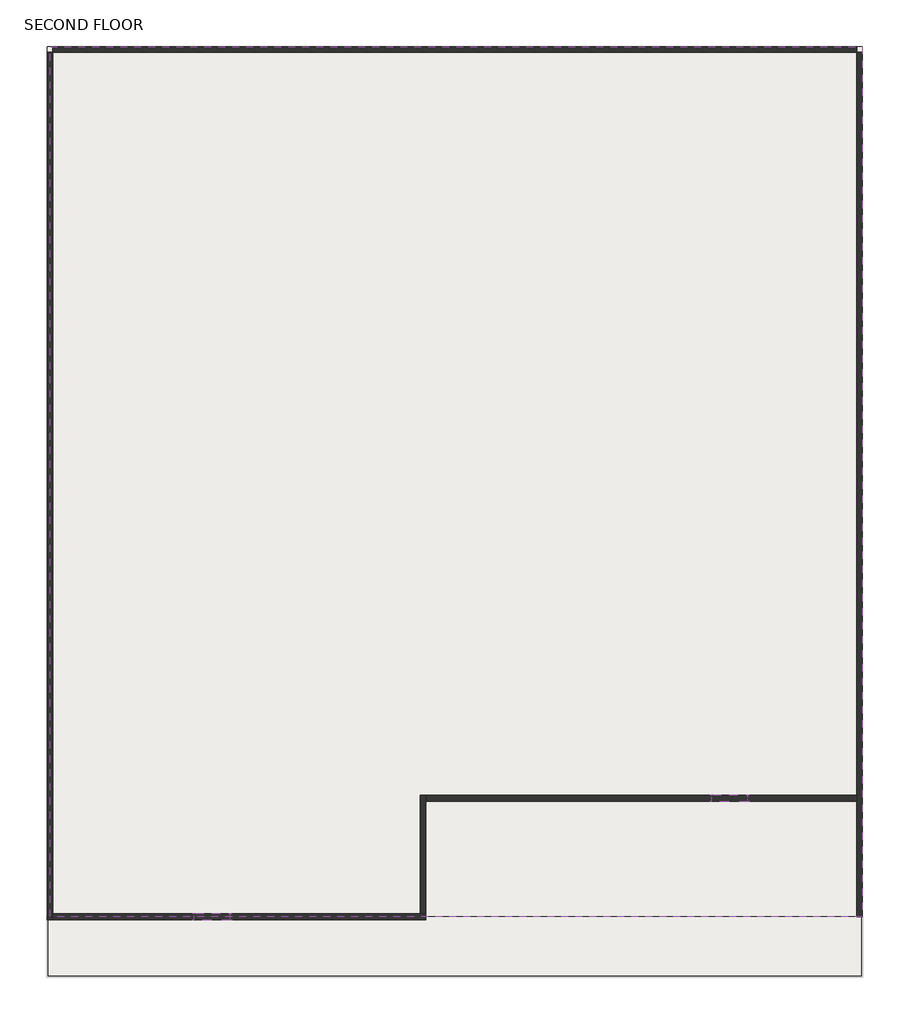
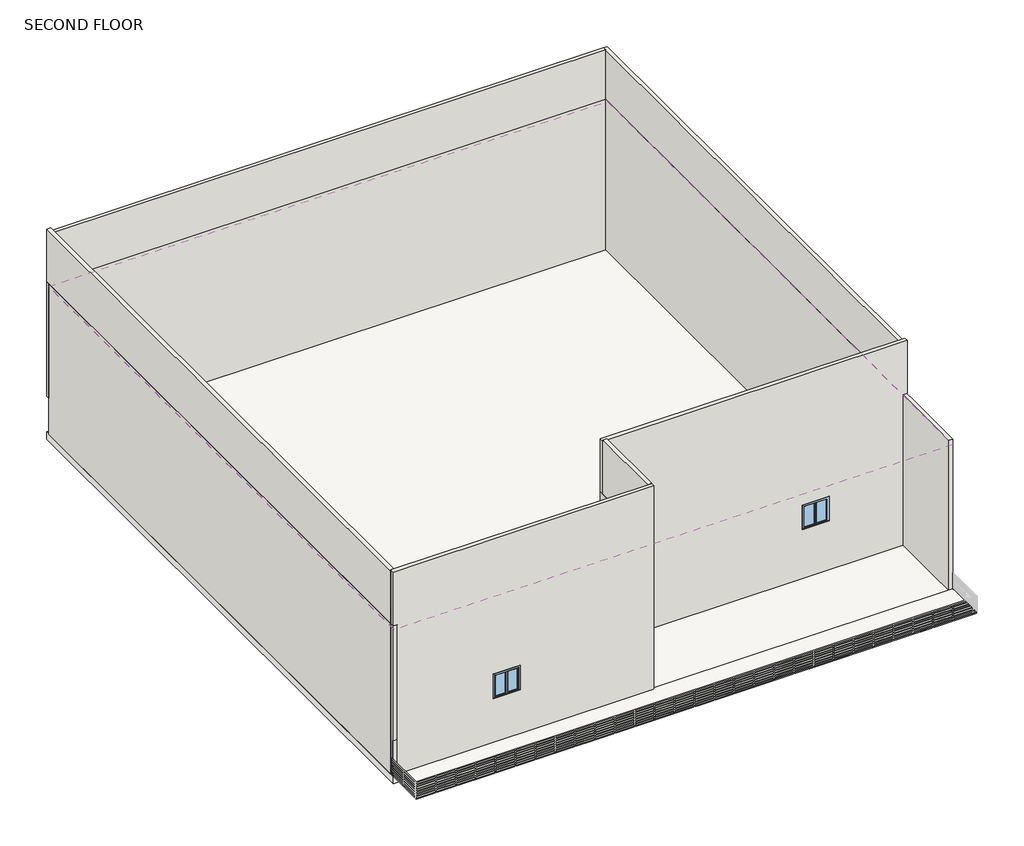
# One storey, part 1 of 2: 13 walls, 3 slabs, 2 coverings, 2 windows.
"""IFC4 building model written with IfcOpenShell, lengths in millimetres."""

from ifc_helpers import new_model, si_unit, frame, origin, place, context, project, spatial, polyline, outline, extrude, faceted_brep, transform, mapped, element, save
from components import window_264d1730

model = new_model("IFC4")

# Units and contexts
model_context = context("Model", 3, world=origin())
ifc_project = project(units=[si_unit("LENGTHUNIT", "METRE", prefix="MILLI")], contexts=[model_context])

# Site, building, storey
site = spatial("IfcSite", under=ifc_project)
building = spatial("IfcBuilding", under=site)
storey = spatial("IfcBuildingStorey", under=building, Name="SECOND FLOOR", Elevation=6096.0)

# Coverings
placement = place(None, origin())
element("IfcCovering", 1, ObjectType="600 x 1200mm grid", at=placement, inside=storey, context=model_context, shape_type="SweptSolid", body=[
    extrude(outline(polyline([(10309.98018, -7832.8965627), (10309.98018, -9913.0763423), (-17890.01982, -9913.0763423), (-17890.01982, -7832.8965627), (10309.98018, -7832.8965627)])), frame((0.0, 0.0, 6096.0), z_axis=(0.0, 0.0, 1.0), x_axis=(1.0, 0.0, 0.0)), (0.0, 0.0, 1.0), 52.0),
])
element("IfcCovering", 2, ObjectType="Generic - 300mm", at=placement, inside=storey, context=model_context, shape_type="SweptSolid", body=[
    extrude(outline(polyline([(10309.98018, 22263.7395992), (10309.98018, -7836.2604008), (-17790.01982, -7836.2604008), (-17790.01982, 22263.7395992), (10309.98018, 22263.7395992)])), frame((0.0, 0.0, 13800.0), z_axis=(0.0, 0.0, 1.0), x_axis=(1.0, 0.0, 0.0)), (0.0, 0.0, 1.0), 300.0),
])

# Slabs
element("IfcSlab", 3, ObjectType="Generic Floor - 400mm", at=placement, inside=storey, context=model_context, shape_type="SweptSolid", body=[
    extrude(outline(polyline([(10309.98018, 22267.1034373), (10309.98018, -7932.8965627), (-17890.01982, -7932.8965627), (-17890.01982, 22267.1034373), (10309.98018, 22267.1034373)])), frame((0.0, 0.0, 5696.0), z_axis=(0.0, 0.0, 1.0), x_axis=(1.0, 0.0, 0.0)), (0.0, 0.0, 1.0), 400.0),
])
element("IfcSlab", 4, ObjectType="Generic Floor - 400mm", at=placement, inside=storey, context=model_context, shape_type="SweptSolid", body=[
    extrude(outline(polyline([(10309.98018, 22267.1034373), (10309.98018, -7932.8965627), (-17890.01982, -7932.8965627), (-17890.01982, 22267.1034373), (10309.98018, 22267.1034373)])), frame((0.0, 0.0, 5696.0), z_axis=(0.0, 0.0, 1.0), x_axis=(1.0, 0.0, 0.0)), (0.0, 0.0, 1.0), 400.0),
])
element("IfcSlab", 5, ObjectType="Generic Floor - 400mm", at=placement, inside=storey, context=model_context, shape_type="SweptSolid", body=[
    extrude(outline(polyline([(10309.98018, 22267.1034373), (10309.98018, -7832.8965627), (-17890.01982, -7832.8965627), (-17890.01982, 22267.1034373), (10309.98018, 22267.1034373)])), frame((0.0, 0.0, 5696.0), z_axis=(0.0, 0.0, 1.0), x_axis=(1.0, 0.0, 0.0)), (0.0, 0.0, 1.0), 400.0),
])

# Walls
element("IfcWall", 6, ObjectType="Generic - 9\"", at=placement, inside=storey, context=model_context, shape_type="Brep", body=[
    faceted_brep([(-17690.01982, 22067.1034373, 6096.0), (10109.98018, 22067.1034373, 6096.0), (10109.98018, 22067.1034373, 14096.0), (-17690.01982, 22067.1034373, 14096.0), (-17890.01982, 22067.1034373, 14096.0), (-17890.01982, 22067.1034373, 8000.0), (-17690.01982, 22067.1034373, 8000.0), (-17690.01982, 22267.1034373, 6096.0), (-17690.01982, 22267.1034373, 8000.0), (-17890.01982, 22267.1034373, 8000.0), (-17890.01982, 22267.1034373, 14096.0), (-17690.01982, 22267.1034373, 14096.0), (10109.98018, 22267.1034373, 14096.0), (10109.98018, 22267.1034373, 8000.0), (10109.98018, 22267.1034373, 6096.0)], [[[0, 1, 2, 3, 4, 5, 6]], [[7, 8, 9, 10, 11, 12, 13, 14]], [[1, 0, 7, 14]], [[4, 3, 2, 12, 11, 10]], [[5, 9, 8, 6]], [[0, 6, 8, 7]], [[5, 4, 10, 9]], [[1, 14, 13, 12, 2]]]),
])
element("IfcWall", 7, ObjectType="Generic - 9\"", at=placement, inside=storey, context=model_context, shape_type="Brep", body=[
    faceted_brep([(-17690.01982, -7832.8965627, 6096.0), (-17690.01982, -7732.8965627, 6096.0), (-17690.01982, 22067.1034373, 6096.0), (-17690.01982, 22067.1034373, 14096.0), (-17690.01982, -7732.8965627, 14096.0), (-17690.01982, -7932.8965627, 14096.0), (-17690.01982, -7932.8965627, 8000.0), (-17690.01982, -7832.8965627, 8000.0), (-17890.01982, -7832.8965627, 6096.0), (-17890.01982, -7832.8965627, 8000.0), (-17890.01982, -7932.8965627, 8000.0), (-17890.01982, -7932.8965627, 14096.0), (-17890.01982, -7732.8965627, 14096.0), (-17890.01982, 22067.1034373, 14096.0), (-17890.01982, 22067.1034373, 8000.0), (-17890.01982, 22067.1034373, 6096.0)], [[[0, 1, 2, 3, 4, 5, 6, 7]], [[8, 9, 10, 11, 12, 13, 14, 15]], [[2, 1, 0, 8, 15]], [[5, 4, 3, 13, 12, 11]], [[2, 15, 14, 13, 3]], [[0, 7, 9, 8]], [[6, 10, 9, 7]], [[6, 5, 11, 10]]]),
])
element("IfcWall", 8, ObjectType="Generic - 9\"", at=placement, inside=storey, context=model_context, shape_type="Brep", body=[
    faceted_brep([(10109.98018, 22067.1034373, 6096.0), (10109.98018, -3632.8965627, 6096.0), (10109.98018, -3832.8965627, 6096.0), (10109.98018, -7832.8965627, 6096.0), (10109.98018, -7832.8965627, 14096.0), (10109.98018, -3832.8965627, 14096.0), (10109.98018, -3632.8965627, 14096.0), (10109.98018, 22067.1034373, 14096.0), (10109.98018, 22267.1034373, 14096.0), (10109.98018, 22267.1034373, 8000.0), (10109.98018, 22067.1034373, 8000.0), (10309.98018, 22067.1034373, 6096.0), (10309.98018, 22067.1034373, 8000.0), (10309.98018, 22267.1034373, 8000.0), (10309.98018, 22267.1034373, 14096.0), (10309.98018, 22067.1034373, 14096.0), (10309.98018, -7832.8965627, 14096.0), (10309.98018, -7832.8965627, 6096.0)], [[[0, 1, 2, 3, 4, 5, 6, 7, 8, 9, 10]], [[11, 12, 13, 14, 15, 16, 17]], [[3, 2, 1, 0, 11, 17]], [[4, 3, 17, 16]], [[8, 7, 6, 5, 4, 16, 15, 14]], [[9, 13, 12, 10]], [[0, 10, 12, 11]], [[9, 8, 14, 13]]]),
])
element("IfcWall", 9, ObjectType="Generic - 9\"", at=placement, inside=storey, context=model_context, shape_type="Brep", body=[
    faceted_brep([(-17690.01982, 22067.1034373, 14096.0), (-17690.01982, 22067.1034373, 6096.0), (10109.98018, 22067.1034373, 6096.0), (10109.98018, 22067.1034373, 14096.0), (-17690.01982, 22267.1034373, 6096.0), (-17690.01982, 22267.1034373, 14096.0), (10109.98018, 22267.1034373, 14096.0), (10109.98018, 22267.1034373, 8000.0), (10109.98018, 22267.1034373, 6096.0)], [[[0, 1, 2, 3]], [[4, 5, 6, 7, 8]], [[2, 1, 4, 8]], [[0, 3, 6, 5]], [[0, 5, 4, 1]], [[2, 8, 7, 6, 3]]]),
])
element("IfcWall", 10, ObjectType="Generic - 9\"", at=placement, inside=storey, context=model_context, shape_type="Brep", body=[
    faceted_brep([(-17690.01982, -7932.8965627, 14096.0), (-17690.01982, -7932.8965627, 6096.0), (-17690.01982, -7832.8965627, 6096.0), (-17690.01982, -7732.8965627, 6096.0), (-17690.01982, 22067.1034373, 6096.0), (-17690.01982, 22067.1034373, 14096.0), (-17690.01982, -7732.8965627, 14096.0), (-17890.01982, -7932.8965627, 6096.0), (-17890.01982, -7932.8965627, 14096.0), (-17890.01982, -7732.8965627, 14096.0), (-17890.01982, 22067.1034373, 14096.0), (-17890.01982, 22067.1034373, 8000.0), (-17890.01982, 22067.1034373, 6096.0), (-17890.01982, -7832.8965627, 6096.0)], [[[0, 1, 2, 3, 4, 5, 6]], [[7, 8, 9, 10, 11, 12, 13]], [[4, 3, 2, 1, 7, 13, 12]], [[0, 6, 5, 10, 9, 8]], [[4, 12, 11, 10, 5]], [[0, 8, 7, 1]]]),
])
element("IfcWall", 11, ObjectType="Generic - 9\"", at=placement, inside=storey, context=model_context, shape_type="Brep", body=[
    faceted_brep([(10109.98018, 22067.1034373, 14096.0), (10109.98018, 22067.1034373, 6096.0), (10109.98018, -3632.8965627, 6096.0), (10109.98018, -3832.8965627, 6096.0), (10109.98018, -7832.8965627, 6096.0), (10109.98018, -7832.8965627, 14096.0), (10109.98018, -3832.8965627, 14096.0), (10109.98018, -3632.8965627, 14096.0), (10309.98018, 22067.1034373, 6096.0), (10309.98018, 22067.1034373, 8000.0), (10309.98018, 22067.1034373, 14096.0), (10309.98018, -7832.8965627, 14096.0), (10309.98018, -7832.8965627, 6096.0)], [[[0, 1, 2, 3, 4, 5, 6, 7]], [[8, 9, 10, 11, 12]], [[4, 3, 2, 1, 8, 12]], [[5, 4, 12, 11]], [[0, 7, 6, 5, 11, 10]], [[0, 10, 9, 8, 1]]]),
])
element("IfcWall", 12, ObjectType="Generic - 9\"", at=placement, inside=storey, context=model_context, shape_type="Brep", body=[
    faceted_brep([(-17690.01982, -7932.8965627, 14096.0), (-17690.01982, -7932.8965627, 8000.0), (-17690.01982, -7932.8965627, 6096.0), (-4790.01982, -7932.8965627, 6096.0), (-4790.01982, -7932.8965627, 16953.9718383), (-17890.01982, -7932.8965627, 16953.9718383), (-17890.01982, -7932.8965627, 14096.0), (-12799.61982, -7932.8965627, 9715.2), (-11580.41982, -7932.8965627, 9715.2), (-11580.41982, -7932.8965627, 8496.0), (-12799.61982, -7932.8965627, 8496.0), (-17690.01982, -7732.8965627, 6096.0), (-17690.01982, -7732.8965627, 14096.0), (-17890.01982, -7732.8965627, 14096.0), (-17890.01982, -7732.8965627, 16885.2976154), (-17890.01982, -7732.8965627, 16953.9718383), (-4790.01982, -7732.8965627, 16953.9718383), (-4790.01982, -7732.8965627, 14096.0), (-4790.01982, -7732.8965627, 6096.0), (-4990.01982, -7732.8965627, 6096.0), (-12799.61982, -7732.8965627, 9715.2), (-12799.61982, -7732.8965627, 8496.0), (-11580.41982, -7732.8965627, 8496.0), (-11580.41982, -7732.8965627, 9715.2), (-17690.01982, -7832.8965627, 6096.0)], [[[0, 1, 2, 3, 4, 5, 6], [7, 8, 9, 10]], [[11, 12, 13, 14, 15, 16, 17, 18, 19], [20, 21, 22, 23]], [[3, 2, 24, 11, 19, 18]], [[5, 4, 16, 15]], [[21, 20, 7, 10]], [[22, 21, 10, 9]], [[23, 22, 9, 8]], [[20, 23, 8, 7]], [[3, 18, 17, 16, 4]], [[6, 13, 12, 0]], [[0, 12, 11, 24, 2, 1]], [[6, 5, 15, 14, 13]]]),
])
element("IfcWall", 13, ObjectType="Generic - 9\"", at=placement, inside=storey, context=model_context, shape_type="Brep", body=[
    faceted_brep([(-4790.01982, -7732.8965627, 6096.0), (-4790.01982, -3832.8965627, 6096.0), (-4790.01982, -3632.8965627, 6096.0), (-4790.01982, -3632.8965627, 14096.0), (-4790.01982, -3832.8965627, 14096.0), (-4790.01982, -7732.8965627, 14096.0), (-4990.01982, -7732.8965627, 6096.0), (-4990.01982, -7732.8965627, 14096.0), (-4990.01982, -3832.8965627, 14096.0), (-4990.01982, -3632.8965627, 14096.0), (-4990.01982, -3632.8965627, 6096.0)], [[[0, 1, 2, 3, 4, 5]], [[6, 7, 8, 9, 10]], [[2, 1, 0, 6, 10]], [[5, 4, 3, 9, 8, 7]], [[0, 5, 7, 6]], [[3, 2, 10, 9]]]),
])
element("IfcWall", 14, ObjectType="Generic - 9\"", at=placement, inside=storey, context=model_context, shape_type="Brep", body=[
    faceted_brep([(-4790.01982, -3832.8965627, 6096.0), (10109.98018, -3832.8965627, 6096.0), (10109.98018, -3832.8965627, 14096.0), (10309.98018, -3832.8965627, 14096.0), (10309.98018, -3832.8965627, 16919.8001369), (-4990.01982, -3832.8965627, 16919.8001369), (-4990.01982, -3832.8965627, 14096.0), (-4790.01982, -3832.8965627, 14096.0), (5100.38018, -3832.8965627, 9942.9261475), (6319.58018, -3832.8965627, 9942.9261475), (6319.58018, -3832.8965627, 8723.7261475), (5100.38018, -3832.8965627, 8723.7261475), (-4790.01982, -3632.8965627, 6096.0), (-4790.01982, -3632.8965627, 14096.0), (-4990.01982, -3632.8965627, 14096.0), (-4990.01982, -3632.8965627, 16919.8001369), (10309.98018, -3632.8965627, 16919.8001369), (10309.98018, -3632.8965627, 16713.0270104), (10309.98018, -3632.8965627, 14096.0), (10109.98018, -3632.8965627, 14096.0), (10109.98018, -3632.8965627, 6096.0), (5100.38018, -3632.8965627, 9942.9261475), (5100.38018, -3632.8965627, 8723.7261475), (6319.58018, -3632.8965627, 8723.7261475), (6319.58018, -3632.8965627, 9942.9261475)], [[[0, 1, 2, 3, 4, 5, 6, 7], [8, 9, 10, 11]], [[12, 13, 14, 15, 16, 17, 18, 19, 20], [21, 22, 23, 24]], [[1, 0, 12, 20]], [[5, 4, 16, 15]], [[22, 21, 8, 11]], [[23, 22, 11, 10]], [[24, 23, 10, 9]], [[21, 24, 9, 8]], [[6, 14, 13, 7]], [[0, 7, 13, 12]], [[6, 5, 15, 14]], [[18, 3, 2, 19]], [[2, 1, 20, 19]], [[4, 3, 18, 17, 16]]]),
])
element("IfcWall", 15, ObjectType="Generic - 9\"", at=placement, inside=storey, context=model_context, shape_type="Brep", body=[
    faceted_brep([(-4990.01982, -3832.8965627, 16963.2919591), (-4990.01982, -3832.8965627, 16919.8001369), (-4990.01982, -3832.8965627, 14096.0), (-4990.01982, -3832.8965627, 6096.0), (-4990.01982, -7732.8965627, 6096.0), (-4990.01982, -7732.8965627, 16963.2919591), (-4790.01982, -3832.8965627, 6096.0), (-4790.01982, -3832.8965627, 16963.2919591), (-4790.01982, -7732.8965627, 16963.2919591), (-4790.01982, -7732.8965627, 16953.9718383), (-4790.01982, -7732.8965627, 6096.0)], [[[0, 1, 2, 3, 4, 5]], [[6, 7, 8, 9, 10]], [[4, 3, 6, 10]], [[0, 5, 8, 7]], [[0, 7, 6, 3, 2, 1]], [[4, 10, 9, 8, 5]]]),
])
element("IfcWall", 16, ObjectType="Generic - 9\"", at=placement, inside=storey, context=model_context, shape_type="Brep", body=[
    faceted_brep([(-17690.01982, -7732.8965627, 16885.2976154), (-17690.01982, -7732.8965627, 6096.0), (-17690.01982, 22067.1034373, 6096.0), (-17690.01982, 22067.1034373, 14096.0), (-17690.01982, 22267.1034373, 14096.0), (-17690.01982, 22267.1034373, 16729.6386618), (-17690.01982, 22267.1034373, 16885.2976154), (-17890.01982, -7732.8965627, 6096.0), (-17890.01982, -7732.8965627, 14096.0), (-17890.01982, -7732.8965627, 16885.2976154), (-17890.01982, 22267.1034373, 16885.2976154), (-17890.01982, 22267.1034373, 14096.0), (-17890.01982, 22067.1034373, 14096.0), (-17890.01982, 22067.1034373, 8000.0), (-17890.01982, 22067.1034373, 6096.0)], [[[0, 1, 2, 3, 4, 5, 6]], [[7, 8, 9, 10, 11, 12, 13, 14]], [[2, 1, 7, 14]], [[0, 6, 10, 9]], [[11, 4, 3, 12]], [[2, 14, 13, 12, 3]], [[6, 5, 4, 11, 10]], [[0, 9, 8, 7, 1]]]),
])
element("IfcWall", 17, ObjectType="Generic - 9\"", at=placement, inside=storey, context=model_context, shape_type="Brep", body=[
    faceted_brep([(10109.98018, 22067.1034373, 14096.0), (10109.98018, 22067.1034373, 6096.0), (10109.98018, -3632.8965627, 6096.0), (10109.98018, -3632.8965627, 16713.0270104), (10109.98018, 22267.1034373, 16713.0270104), (10109.98018, 22267.1034373, 14096.0), (10309.98018, 22067.1034373, 6096.0), (10309.98018, 22067.1034373, 8000.0), (10309.98018, 22067.1034373, 14096.0), (10309.98018, 22267.1034373, 14096.0), (10309.98018, 22267.1034373, 16713.0270104), (10309.98018, -3632.8965627, 16713.0270104), (10309.98018, -3632.8965627, 14096.0), (10309.98018, -3632.8965627, 6096.0)], [[[0, 1, 2, 3, 4, 5]], [[6, 7, 8, 9, 10, 11, 12, 13]], [[2, 1, 6, 13]], [[4, 3, 11, 10]], [[3, 2, 13, 12, 11]], [[5, 9, 8, 0]], [[0, 8, 7, 6, 1]], [[5, 4, 10, 9]]]),
])
element("IfcWall", 18, ObjectType="Generic - 9\"", at=placement, inside=storey, context=model_context, shape_type="Brep", body=[
    faceted_brep([(10109.98018, 22267.1034373, 16729.6386618), (10109.98018, 22267.1034373, 16713.0270104), (10109.98018, 22267.1034373, 14096.0), (10109.98018, 22267.1034373, 8000.0), (10109.98018, 22267.1034373, 6096.0), (-17690.01982, 22267.1034373, 6096.0), (-17690.01982, 22267.1034373, 14096.0), (-17690.01982, 22267.1034373, 16729.6386618), (10109.98018, 22067.1034373, 6096.0), (10109.98018, 22067.1034373, 16729.6386618), (-17690.01982, 22067.1034373, 16729.6386618), (-17690.01982, 22067.1034373, 6096.0)], [[[0, 1, 2, 3, 4, 5, 6, 7]], [[8, 9, 10, 11]], [[5, 4, 8, 11]], [[0, 7, 10, 9]], [[0, 9, 8, 4, 3, 2, 1]], [[5, 11, 10, 7, 6]]]),
])

# Windows
window_shape = window_264d1730(model_context)
element("IfcWindow", 19, ObjectType="Casement Dbl with Trim : 48\" x 48\"", at=placement, inside=storey, context=model_context, shape_type="MappedRepresentation", body=[
    mapped(window_shape, transform((5709.98018, -3713.8465627, 7809.3261475), x_axis=(-1.0, 0.0, 0.0), y_axis=(0.0, -1.0, 0.0), z_axis=(0.0, 0.0, 1.0))),
])
element("IfcWindow", 20, ObjectType="Casement Dbl with Trim : 48\" x 48\"", at=placement, inside=storey, context=model_context, shape_type="MappedRepresentation", body=[
    mapped(window_shape, transform((-12190.01982, -7813.8465627, 7581.6), x_axis=(-1.0, 0.0, 0.0), y_axis=(0.0, -1.0, 0.0), z_axis=(0.0, 0.0, 1.0))),
])

save(model, "model.ifc")

# Revit data of these elements
# Type "600 x 1200mm grid"
#   built-in parameter 1002203 = 1 (stored number, unit not read)
#   built-in parameter 1002202 = 1 (stored number, unit not read)
#   Layers, outside or top first: 0' - 1.41732" "Default" (function 1); 0' - 0.62992" "Ceiling Tile 600 x 1200" (function 5)
# Type "Generic - 300mm"
#   built-in parameter 1002203 = 1 (stored number, unit not read)
#   built-in parameter 1002202 = 1 (stored number, unit not read)
#   Layers, outside or top first: 0' - 11.81102" no material (function 1)
# Type "Generic Floor - 400mm"
#   Function = 0
#   Layers, outside or top first: 1' - 3.74803" no material (function 1)
# Type "Generic - 9\""
#   Layers, outside or top first: 0' - 7.87402" no material (function 1)
# Type "Casement Dbl with Trim : 48\" x 48\""
#   Type Mark = "19"
#   Construction Type Id = "GSP4R"
#   Assembly Code = "B2020100"
#   Analytic Construction = "1/8 in Pilkington single glazing"
#   Visual Light Transmittance = 0.9
#   Solar Heat Gain Coefficient = 0.78
#   Heat Transfer Coefficient (U) = 3.6886 W/(m²·K)
#   Height = 4' - 0"
#   Default Sill Height = 3' - 0"
#   Trim Projection - Ext. = 0' - 0 1/2"
#   Trim Projection - Int. = 0' - 0 3/4"
#   Trim Width - Exterior = 0' - 3 1/2"
#   Trim Width - Interior = 0' - 3 1/2"
#   Width = 4' - 0"
#   Window Inset = 0' - 0 3/4"
#   Define Thermal Properties by = 1
#   Glass Pane Material = Glass
#   Sash Material = Sash
#   Trim Exterior Material = Trim
#   Trim Interior Material = Trim
#   Wall Closure = (empty or 0)
# Element 1 (IfcCovering, "600 x 1200mm grid")
#   Height Offset From Level = 0' - 0"
#   Phase Created = New Construction
#   Materials on its faces: "Ceiling Tile 600 x 1200", "Default"
# Element 2 (IfcCovering, "Generic - 300mm")
#   Height Offset From Level = 25' - 3.30709"
#   Phase Created = New Construction
#   Materials on its faces: "Default Roof"
# Elements 3, 4, 5 (IfcSlab, "Generic Floor - 400mm")
#   Height Offset From Level = 0' - 0"
#   Phase Created = New Construction
#   Materials on its faces: "Default Roof"
# Elements 6, 7, 8, 9, 10, 11, 13 (IfcWall, "Generic - 9\"")
#   Top Offset = 0' - 0"
#   Base Offset = 0' - 0"
#   Unconnected Height = 26' - 2.96063"
#   wall height = 26' - 2.96063"
#   Phase Created = New Construction
#   Base Constraint = SECOND FLOOR
#   Materials on its faces: "Default Wall"
# Element 12 (IfcWall, "Generic - 9\"")
#   Top Offset = 0' - 0"
#   Base Offset = 0' - 0"
#   Unconnected Height = 35' - 7.47921"
#   wall height = 35' - 7.47921"
#   Phase Created = New Construction
#   Base Constraint = SECOND FLOOR
#   Materials on its faces: "Default Wall"
# Element 14 (IfcWall, "Generic - 9\"")
#   Top Offset = 0' - 0"
#   Base Offset = 0' - 0"
#   Unconnected Height = 35' - 6.13386"
#   wall height = 35' - 6.13386"
#   Phase Created = New Construction
#   Base Constraint = SECOND FLOOR
#   Materials on its faces: "Default Wall"
# Element 15 (IfcWall, "Generic - 9\"")
#   Top Offset = 0' - 0"
#   Base Offset = 0' - 0"
#   Unconnected Height = 35' - 7.84614"
#   wall height = 35' - 7.84614"
#   Phase Created = New Construction
#   Base Constraint = SECOND FLOOR
#   Materials on its faces: "Default Wall"
# Element 16 (IfcWall, "Generic - 9\"")
#   Top Offset = 0' - 0"
#   Base Offset = 0' - 0"
#   Unconnected Height = 35' - 4.7755"
#   wall height = 35' - 4.7755"
#   Phase Created = New Construction
#   Base Constraint = SECOND FLOOR
#   Materials on its faces: "Default Wall"
# Element 17 (IfcWall, "Generic - 9\"")
#   Top Offset = 0' - 0"
#   Base Offset = 0' - 0"
#   Unconnected Height = 34' - 9.99319"
#   wall height = 34' - 9.99319"
#   Phase Created = New Construction
#   Base Constraint = SECOND FLOOR
#   Materials on its faces: "Default Wall"
# Element 18 (IfcWall, "Generic - 9\"")
#   Top Offset = 0' - 0"
#   Base Offset = 0' - 0"
#   Unconnected Height = 34' - 10.64719"
#   wall height = 34' - 10.64719"
#   Phase Created = New Construction
#   Base Constraint = SECOND FLOOR
#   Materials on its faces: "Default Wall"
# Element 19 (IfcWindow, "Casement Dbl with Trim : 48\" x 48\"")
#   Mark = "10"
#   Phase Created = New Construction
#   Materials on its faces: "Sash", "Trim", "Glass"
# Element 20 (IfcWindow, "Casement Dbl with Trim : 48\" x 48\"")
#   Mark = "11"
#   Phase Created = New Construction
#   Materials on its faces: "Sash", "Trim", "Glass"
# Materials
#   "Default": colour RGB 80 80 80, transparency 0
#   "Ceiling Tile 600 x 1200": class "Generic", colour RGB 179 178 175, transparency 0, Description = "Acoustic ceiling tile", Cost = 0
#   "Glass": class "Glass", colour RGB 218 227 224, transparency 0.85, Description = "Soda Lime Glass", Cost = 0
#   "Sash": class "Wood", colour RGB 136 99 55, transparency 0
#   "Trim": class "Wood", colour RGB 224 178 126, transparency 0
#   "Default Roof": colour RGB 80 80 80, transparency 0
#   "Default Wall": colour RGB 80 80 80, transparency 0
